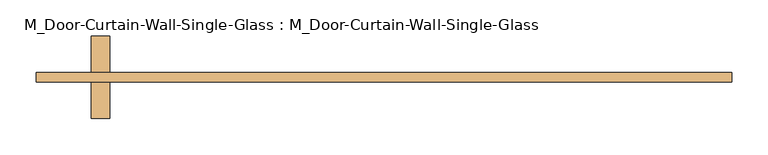
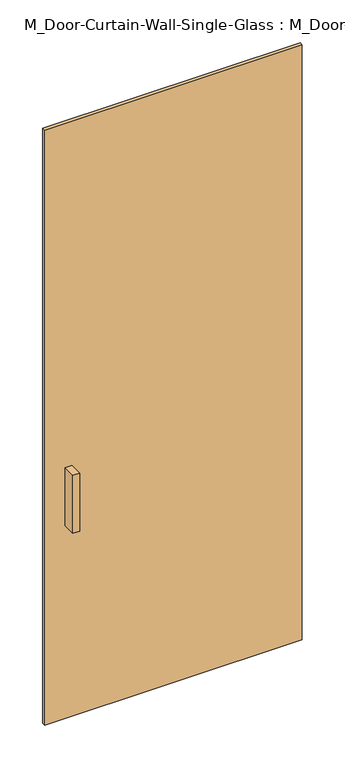
"""IFC4 building model written with IfcOpenShell, lengths in millimetres: door geometry, M_Door-Curtain-Wall-Single-Glass : M_Door-Curtain-Wall-Single-Glass."""

from ifc_helpers import new_model, si_unit, frame, origin, origin_with_axes, place, context, project, spatial, polyline, outline, extrude, source, transform, mapped, element, save


def m_door_curtain_wall_single_glass_m_door_curtain_wall_single_92f462ab(model_context):
    return source(origin(), model_context, "Body", "SweptSolid", [
        extrude(outline(polyline([(481.2500001, -50.8), (-481.2500001, -50.8), (-481.2500001, -38.1), (481.2500001, -38.1), (481.2500001, -50.8)])), origin_with_axes(), (0.0, 0.0, 1.0), 2350.0),
        extrude(outline(polyline([(-405.0500001, -101.6), (-405.0500001, -50.8), (-379.6500001, -50.8), (-379.6500001, -101.6), (-405.0500001, -101.6)])), frame((0.0, 0.0, 762.0), z_axis=(0.0, 0.0, 1.0), x_axis=(1.0, 0.0, 0.0)), (0.0, 0.0, 1.0), 228.6),
        extrude(outline(polyline([(-379.6500001, 12.7), (-379.6500001, -38.1), (-405.0500001, -38.1), (-405.0500001, 12.7), (-379.6500001, 12.7)])), frame((0.0, 0.0, 762.0), z_axis=(0.0, 0.0, 1.0), x_axis=(1.0, 0.0, 0.0)), (0.0, 0.0, 1.0), 228.6),
    ])


if __name__ == "__main__":
    model = new_model("IFC4")
    model_context = context("Model", 3, world=origin())
    ifc_project = project(units=[si_unit("LENGTHUNIT", "METRE", prefix="MILLI")], contexts=[model_context])
    site = spatial("IfcSite", under=ifc_project)
    building = spatial("IfcBuilding", under=site)
    placement = place(None, origin())
    m_door_curtain_wall_single_glass_m_door_curtain_wall_single_shape = m_door_curtain_wall_single_glass_m_door_curtain_wall_single_92f462ab(model_context)
    element("IfcDoor", 1, ObjectType="M_Door-Curtain-Wall-Single-Glass : M_Door-Curtain-Wall-Single-Glass", at=placement, inside=building, context=model_context, shape_type="MappedRepresentation", body=[
        mapped(m_door_curtain_wall_single_glass_m_door_curtain_wall_single_shape, transform((0.0, 0.0, 0.0), x_axis=(1.0, 0.0, 0.0), y_axis=(0.0, 1.0, 0.0), z_axis=(0.0, 0.0, 1.0))),
    ])
    save(model, "model.ifc")

# Revit data of these elements
# Type "M_Door-Curtain-Wall-Single-Glass : M_Door-Curtain-Wall-Single-Glass"
#   Type Mark = "46"
#   Assembly Code = "B2030100"
#   Analytic Construction = "<None>"
#   Width [instance default] = 900 mm
#   Thermal Resistance (R) = 1.7611 (m²·K)/W
#   Swing Angle [instance default] = 90.00°
#   Heat Transfer Coefficient (U) = 0.567826 W/(m²·K)
#   Offset = 50.8 mm
#   Define Thermal Properties by = 1
#   Function = 1
#   Door Handle Material = Aluminum
#   Glazing = Glass
#   Visual Light Transmittance = 0
#   Solar Heat Gain Coefficient = 0
#   Construction Type Id = ""
# Element 1 (IfcDoor, "M_Door-Curtain-Wall-Single-Glass : M_Door-Curtain-Wall-Single-Glass")
#   Width = 962.5 mm
#   Materials on its faces: "Aluminum", "Glass"
# Materials
#   "Aluminum": class "Metal", colour RGB 247 247 247, transparency 0, Description = "Aluminum 6061", Cost = 0
#   "Glass": class "Glass", colour RGB 0 128 192, transparency 0.9, Description = "Soda Lime Glass", Cost = 0
